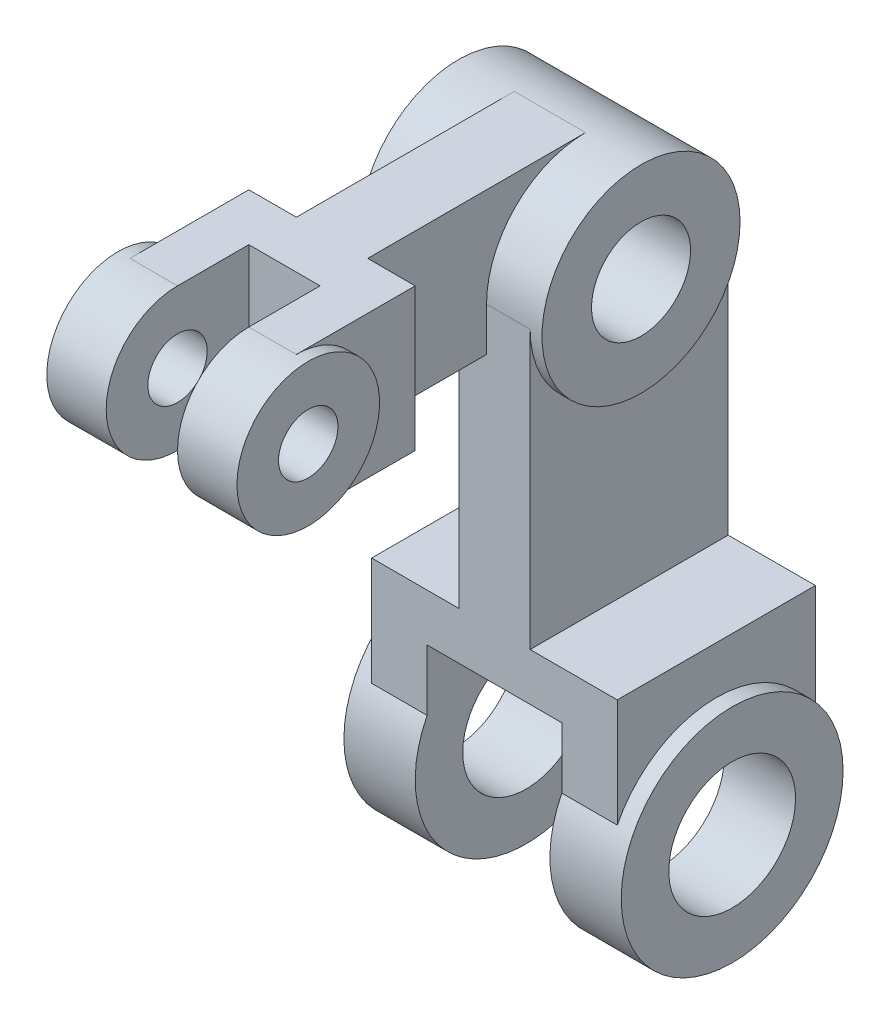
ISO-10303-21;
HEADER;
FILE_DESCRIPTION(('STEP AP214'),'2;1');
FILE_NAME('part.step','',(''),(''),'','','');
FILE_SCHEMA(('AUTOMOTIVE_DESIGN { 1 0 10303 214 1 1 1 1 }'));
ENDSEC;
DATA;
#1=APPLICATION_CONTEXT('core data for automotive mechanical design processes');
#2=APPLICATION_PROTOCOL_DEFINITION('international standard','automotive_design',2000,#1);
#3=PRODUCT_CONTEXT('',#1,'mechanical');
#4=PRODUCT('Part','Part','',(#3));
#5=PRODUCT_RELATED_PRODUCT_CATEGORY('part','',(#4));
#6=PRODUCT_DEFINITION_FORMATION('','',#4);
#7=PRODUCT_DEFINITION_CONTEXT('part definition',#1,'design');
#8=PRODUCT_DEFINITION('design','',#6,#7);
#9=PRODUCT_DEFINITION_SHAPE('','',#8);
#10=(LENGTH_UNIT() NAMED_UNIT(*) SI_UNIT(.MILLI.,.METRE.));
#11=(NAMED_UNIT(*) PLANE_ANGLE_UNIT() SI_UNIT($,.RADIAN.));
#12=(NAMED_UNIT(*) SI_UNIT($,.STERADIAN.) SOLID_ANGLE_UNIT());
#13=UNCERTAINTY_MEASURE_WITH_UNIT(LENGTH_MEASURE(1.E-05),#10,'distance_accuracy_value','');
#14=(GEOMETRIC_REPRESENTATION_CONTEXT(3) GLOBAL_UNCERTAINTY_ASSIGNED_CONTEXT((#13)) GLOBAL_UNIT_ASSIGNED_CONTEXT((#10,
#11,#12)) REPRESENTATION_CONTEXT('',''));
#15=CARTESIAN_POINT('',(0.,0.,0.));
#16=DIRECTION('',(0.,0.,1.));
#17=DIRECTION('',(1.,0.,0.));
#18=AXIS2_PLACEMENT_3D('',#15,#16,#17);
#19=CARTESIAN_POINT('',(-4.,40.,0.));
#20=DIRECTION('',(0.,1.,0.));
#21=DIRECTION('',(0.,0.,1.));
#22=AXIS2_PLACEMENT_3D('',#19,#20,#21);
#23=PLANE('',#22);
#24=DIRECTION('',(-1.,0.,0.));
#25=VECTOR('',#24,1.);
#26=CARTESIAN_POINT('',(-4.,40.,-25.));
#27=LINE('',#26,#25);
#28=CARTESIAN_POINT('',(-4.,40.,-25.));
#29=VERTEX_POINT('',#28);
#30=CARTESIAN_POINT('',(-26.,40.,-25.));
#31=VERTEX_POINT('',#30);
#32=EDGE_CURVE('E366',#29,#31,#27,.T.);
#33=ORIENTED_EDGE('',*,*,#32,.T.);
#34=DIRECTION('',(0.,0.,1.));
#35=VECTOR('',#34,1.);
#36=CARTESIAN_POINT('',(-26.,40.,-25.));
#37=LINE('',#36,#35);
#38=CARTESIAN_POINT('',(-26.,40.,25.));
#39=VERTEX_POINT('',#38);
#40=EDGE_CURVE('E286',#31,#39,#37,.T.);
#41=ORIENTED_EDGE('',*,*,#40,.T.);
#42=DIRECTION('',(-1.,0.,0.));
#43=VECTOR('',#42,1.);
#44=CARTESIAN_POINT('',(-4.,40.,25.));
#45=LINE('',#44,#43);
#46=CARTESIAN_POINT('',(-4.,40.,25.));
#47=VERTEX_POINT('',#46);
#48=EDGE_CURVE('E351',#47,#39,#45,.T.);
#49=ORIENTED_EDGE('',*,*,#48,.F.);
#50=DIRECTION('',(0.,0.,-1.));
#51=VECTOR('',#50,1.);
#52=CARTESIAN_POINT('',(-4.,40.,0.));
#53=LINE('',#52,#51);
#54=EDGE_CURVE('E344',#47,#29,#53,.T.);
#55=ORIENTED_EDGE('',*,*,#54,.T.);
#56=EDGE_LOOP('',(#33,#41,#49,#55));
#57=FACE_BOUND('',#56,.T.);
#58=ADVANCED_FACE('F44',(#57),#23,.T.);
#59=CARTESIAN_POINT('',(-18.,0.,0.));
#60=DIRECTION('',(1.,0.,0.));
#61=DIRECTION('',(0.,0.,-1.));
#62=AXIS2_PLACEMENT_3D('',#59,#60,#61);
#63=CYLINDRICAL_SURFACE('',#62,28.);
#64=DIRECTION('',(-1.,0.,0.));
#65=VECTOR('',#64,1.);
#66=CARTESIAN_POINT('',(-4.,12.6095202129185,25.));
#67=LINE('',#66,#65);
#68=CARTESIAN_POINT('',(-4.,12.6095202129185,25.));
#69=VERTEX_POINT('',#68);
#70=CARTESIAN_POINT('',(-18.,12.6095202129185,25.));
#71=VERTEX_POINT('',#70);
#72=EDGE_CURVE('E359',#69,#71,#67,.T.);
#73=ORIENTED_EDGE('',*,*,#72,.T.);
#74=CARTESIAN_POINT('',(-18.,0.,0.));
#75=DIRECTION('',(1.,0.,0.));
#76=DIRECTION('',(0.,0.,-1.));
#77=AXIS2_PLACEMENT_3D('',#74,#75,#76);
#78=CIRCLE('',#77,28.);
#79=CARTESIAN_POINT('',(-18.,12.6095202129185,-25.));
#80=VERTEX_POINT('',#79);
#81=EDGE_CURVE('E367',#71,#80,#78,.T.);
#82=ORIENTED_EDGE('',*,*,#81,.T.);
#83=DIRECTION('',(-1.,0.,0.));
#84=VECTOR('',#83,1.);
#85=CARTESIAN_POINT('',(-4.,12.6095202129185,-25.));
#86=LINE('',#85,#84);
#87=CARTESIAN_POINT('',(-4.,12.6095202129185,-25.));
#88=VERTEX_POINT('',#87);
#89=EDGE_CURVE('E361',#88,#80,#86,.T.);
#90=ORIENTED_EDGE('',*,*,#89,.F.);
#91=CARTESIAN_POINT('',(-4.,0.,0.));
#92=DIRECTION('',(1.,0.,0.));
#93=DIRECTION('',(0.,0.,1.));
#94=AXIS2_PLACEMENT_3D('',#91,#92,#93);
#95=CIRCLE('',#94,28.);
#96=EDGE_CURVE('E346',#88,#69,#95,.T.);
#97=ORIENTED_EDGE('',*,*,#96,.T.);
#98=EDGE_LOOP('',(#73,#82,#90,#97));
#99=FACE_BOUND('',#98,.T.);
#100=CARTESIAN_POINT('',(0.,0.,0.));
#101=DIRECTION('',(1.,0.,0.));
#102=DIRECTION('',(0.,0.,-1.));
#103=AXIS2_PLACEMENT_3D('',#100,#101,#102);
#104=CIRCLE('',#103,28.);
#105=CARTESIAN_POINT('',(0.,0.,-28.));
#106=VERTEX_POINT('',#105);
#107=EDGE_CURVE('E356',#106,#106,#104,.T.);
#108=ORIENTED_EDGE('',*,*,#107,.F.);
#109=EDGE_LOOP('',(#108));
#110=FACE_BOUND('',#109,.T.);
#111=ADVANCED_FACE('F50',(#99,#110),#63,.T.);
#112=CARTESIAN_POINT('',(-18.,0.,0.));
#113=DIRECTION('',(1.,0.,0.));
#114=DIRECTION('',(0.,0.,-1.));
#115=AXIS2_PLACEMENT_3D('',#112,#113,#114);
#116=PLANE('',#115);
#117=CARTESIAN_POINT('',(-18.,0.,0.));
#118=DIRECTION('',(1.,0.,0.));
#119=DIRECTION('',(0.,0.,-1.));
#120=AXIS2_PLACEMENT_3D('',#117,#118,#119);
#121=CIRCLE('',#120,16.);
#122=CARTESIAN_POINT('',(-18.,0.,-16.));
#123=VERTEX_POINT('',#122);
#124=EDGE_CURVE('E234',#123,#123,#121,.T.);
#125=ORIENTED_EDGE('',*,*,#124,.T.);
#126=EDGE_LOOP('',(#125));
#127=FACE_BOUND('',#126,.T.);
#128=ORIENTED_EDGE('',*,*,#81,.F.);
#129=DIRECTION('',(0.,1.,0.));
#130=VECTOR('',#129,1.);
#131=CARTESIAN_POINT('',(-18.,28.,25.));
#132=LINE('',#131,#130);
#133=CARTESIAN_POINT('',(-18.,28.,25.));
#134=VERTEX_POINT('',#133);
#135=EDGE_CURVE('E303',#71,#134,#132,.T.);
#136=ORIENTED_EDGE('',*,*,#135,.T.);
#137=DIRECTION('',(0.,0.,1.));
#138=VECTOR('',#137,1.);
#139=CARTESIAN_POINT('',(-18.,28.,-40.));
#140=LINE('',#139,#138);
#141=CARTESIAN_POINT('',(-18.,28.,-25.));
#142=VERTEX_POINT('',#141);
#143=EDGE_CURVE('E307',#142,#134,#140,.T.);
#144=ORIENTED_EDGE('',*,*,#143,.F.);
#145=DIRECTION('',(0.,-1.,0.));
#146=VECTOR('',#145,1.);
#147=CARTESIAN_POINT('',(-18.,40.,-25.));
#148=LINE('',#147,#146);
#149=EDGE_CURVE('E375',#142,#80,#148,.T.);
#150=ORIENTED_EDGE('',*,*,#149,.T.);
#151=EDGE_LOOP('',(#128,#136,#144,#150));
#152=FACE_BOUND('',#151,.T.);
#153=ADVANCED_FACE('F505',(#127,#152),#116,.F.);
#154=CARTESIAN_POINT('',(0.,0.,0.));
#155=DIRECTION('',(1.,0.,0.));
#156=DIRECTION('',(0.,0.,-1.));
#157=AXIS2_PLACEMENT_3D('',#154,#155,#156);
#158=PLANE('',#157);
#159=CARTESIAN_POINT('',(0.,0.,0.));
#160=DIRECTION('',(1.,0.,0.));
#161=DIRECTION('',(0.,0.,-1.));
#162=AXIS2_PLACEMENT_3D('',#159,#160,#161);
#163=CIRCLE('',#162,16.);
#164=CARTESIAN_POINT('',(0.,0.,-16.));
#165=VERTEX_POINT('',#164);
#166=EDGE_CURVE('E390',#165,#165,#163,.T.);
#167=ORIENTED_EDGE('',*,*,#166,.F.);
#168=EDGE_LOOP('',(#167));
#169=FACE_BOUND('',#168,.T.);
#170=ORIENTED_EDGE('',*,*,#107,.T.);
#171=EDGE_LOOP('',(#170));
#172=FACE_BOUND('',#171,.T.);
#173=ADVANCED_FACE('F570',(#169,#172),#158,.T.);
#174=DIRECTION('',(0.,0.,1.));
#175=VECTOR('',#174,1.);
#176=CARTESIAN_POINT('',(-44.,40.,-25.));
#177=LINE('',#176,#175);
#178=CARTESIAN_POINT('',(-44.,40.,-25.));
#179=VERTEX_POINT('',#178);
#180=CARTESIAN_POINT('',(-44.,40.,25.));
#181=VERTEX_POINT('',#180);
#182=EDGE_CURVE('E298',#179,#181,#177,.T.);
#183=ORIENTED_EDGE('',*,*,#182,.F.);
#184=CARTESIAN_POINT('',(-66.,40.,-25.));
#185=VERTEX_POINT('',#184);
#186=EDGE_CURVE('E355',#179,#185,#27,.T.);
#187=ORIENTED_EDGE('',*,*,#186,.T.);
#188=DIRECTION('',(0.,0.,-1.));
#189=VECTOR('',#188,1.);
#190=CARTESIAN_POINT('',(-66.,40.,0.));
#191=LINE('',#190,#189);
#192=CARTESIAN_POINT('',(-66.,40.,25.));
#193=VERTEX_POINT('',#192);
#194=EDGE_CURVE('E333',#193,#185,#191,.T.);
#195=ORIENTED_EDGE('',*,*,#194,.F.);
#196=EDGE_CURVE('E360',#181,#193,#45,.T.);
#197=ORIENTED_EDGE('',*,*,#196,.F.);
#198=EDGE_LOOP('',(#183,#187,#195,#197));
#199=FACE_BOUND('',#198,.T.);
#200=ADVANCED_FACE('F521',(#199),#23,.T.);
#201=CARTESIAN_POINT('',(-4.,40.,25.));
#202=DIRECTION('',(0.,0.,1.));
#203=DIRECTION('',(1.,0.,0.));
#204=AXIS2_PLACEMENT_3D('',#201,#202,#203);
#205=PLANE('',#204);
#206=DIRECTION('',(0.,1.,0.));
#207=VECTOR('',#206,1.);
#208=CARTESIAN_POINT('',(-37.,40.,25.));
#209=LINE('',#208,#207);
#210=CARTESIAN_POINT('',(-37.,99.,25.));
#211=VERTEX_POINT('',#210);
#212=CARTESIAN_POINT('',(-37.,110.,25.));
#213=VERTEX_POINT('',#212);
#214=EDGE_CURVE('E65',#211,#213,#209,.T.);
#215=ORIENTED_EDGE('',*,*,#214,.F.);
#216=DIRECTION('',(1.,0.,0.));
#217=VECTOR('',#216,1.);
#218=CARTESIAN_POINT('',(-4.,99.,25.));
#219=LINE('',#218,#217);
#220=CARTESIAN_POINT('',(-44.,99.,25.));
#221=VERTEX_POINT('',#220);
#222=EDGE_CURVE('E67',#221,#211,#219,.T.);
#223=ORIENTED_EDGE('',*,*,#222,.F.);
#224=DIRECTION('',(0.,-1.,0.));
#225=VECTOR('',#224,1.);
#226=CARTESIAN_POINT('',(-44.,110.,25.));
#227=LINE('',#226,#225);
#228=EDGE_CURVE('E283',#221,#181,#227,.T.);
#229=ORIENTED_EDGE('',*,*,#228,.T.);
#230=ORIENTED_EDGE('',*,*,#196,.T.);
#231=DIRECTION('',(0.,1.,0.));
#232=VECTOR('',#231,1.);
#233=CARTESIAN_POINT('',(-66.,40.,25.));
#234=LINE('',#233,#232);
#235=CARTESIAN_POINT('',(-66.,12.6095202129185,25.));
#236=VERTEX_POINT('',#235);
#237=EDGE_CURVE('E338',#236,#193,#234,.T.);
#238=ORIENTED_EDGE('',*,*,#237,.F.);
#239=DIRECTION('',(1.,0.,0.));
#240=VECTOR('',#239,1.);
#241=CARTESIAN_POINT('',(-70.,12.6095202129185,25.));
#242=LINE('',#241,#240);
#243=CARTESIAN_POINT('',(-52.,12.6095202129185,25.));
#244=VERTEX_POINT('',#243);
#245=EDGE_CURVE('E329',#236,#244,#242,.T.);
#246=ORIENTED_EDGE('',*,*,#245,.T.);
#247=DIRECTION('',(0.,-1.,0.));
#248=VECTOR('',#247,1.);
#249=CARTESIAN_POINT('',(-52.,12.6095202129185,25.));
#250=LINE('',#249,#248);
#251=CARTESIAN_POINT('',(-52.,28.,25.));
#252=VERTEX_POINT('',#251);
#253=EDGE_CURVE('E299',#252,#244,#250,.T.);
#254=ORIENTED_EDGE('',*,*,#253,.F.);
#255=DIRECTION('',(-1.,0.,0.));
#256=VECTOR('',#255,1.);
#257=CARTESIAN_POINT('',(-52.,28.,25.));
#258=LINE('',#257,#256);
#259=EDGE_CURVE('E306',#134,#252,#258,.T.);
#260=ORIENTED_EDGE('',*,*,#259,.F.);
#261=ORIENTED_EDGE('',*,*,#135,.F.);
#262=ORIENTED_EDGE('',*,*,#72,.F.);
#263=DIRECTION('',(0.,1.,0.));
#264=VECTOR('',#263,1.);
#265=CARTESIAN_POINT('',(-4.,40.,25.));
#266=LINE('',#265,#264);
#267=EDGE_CURVE('E353',#69,#47,#266,.T.);
#268=ORIENTED_EDGE('',*,*,#267,.T.);
#269=ORIENTED_EDGE('',*,*,#48,.T.);
#270=DIRECTION('',(0.,1.,0.));
#271=VECTOR('',#270,1.);
#272=CARTESIAN_POINT('',(-26.,40.,25.));
#273=LINE('',#272,#271);
#274=CARTESIAN_POINT('',(-26.,110.,25.));
#275=VERTEX_POINT('',#274);
#276=EDGE_CURVE('E282',#39,#275,#273,.T.);
#277=ORIENTED_EDGE('',*,*,#276,.T.);
#278=DIRECTION('',(-1.,0.,0.));
#279=VECTOR('',#278,1.);
#280=CARTESIAN_POINT('',(-26.,110.,25.));
#281=LINE('',#280,#279);
#282=EDGE_CURVE('E291',#275,#213,#281,.T.);
#283=ORIENTED_EDGE('',*,*,#282,.T.);
#284=EDGE_LOOP('',(#215,#223,#229,#230,#238,#246,#254,#260,#261,#262,#268,#269,#277,#283));
#285=FACE_BOUND('',#284,.T.);
#286=ADVANCED_FACE('F483',(#285),#205,.T.);
#287=CARTESIAN_POINT('',(-4.,40.,-25.));
#288=DIRECTION('',(0.,0.,-1.));
#289=DIRECTION('',(-1.,0.,0.));
#290=AXIS2_PLACEMENT_3D('',#287,#288,#289);
#291=PLANE('',#290);
#292=DIRECTION('',(0.,1.,0.));
#293=VECTOR('',#292,1.);
#294=CARTESIAN_POINT('',(-52.,40.,-25.));
#295=LINE('',#294,#293);
#296=CARTESIAN_POINT('',(-52.,12.6095202129185,-25.));
#297=VERTEX_POINT('',#296);
#298=CARTESIAN_POINT('',(-52.,28.,-25.));
#299=VERTEX_POINT('',#298);
#300=EDGE_CURVE('E317',#297,#299,#295,.T.);
#301=ORIENTED_EDGE('',*,*,#300,.F.);
#302=DIRECTION('',(1.,0.,0.));
#303=VECTOR('',#302,1.);
#304=CARTESIAN_POINT('',(-70.,12.6095202129185,-25.));
#305=LINE('',#304,#303);
#306=CARTESIAN_POINT('',(-66.,12.6095202129185,-25.));
#307=VERTEX_POINT('',#306);
#308=EDGE_CURVE('E324',#297,#307,#305,.F.);
#309=ORIENTED_EDGE('',*,*,#308,.T.);
#310=DIRECTION('',(0.,-1.,0.));
#311=VECTOR('',#310,1.);
#312=CARTESIAN_POINT('',(-66.,40.,-25.));
#313=LINE('',#312,#311);
#314=EDGE_CURVE('E335',#185,#307,#313,.T.);
#315=ORIENTED_EDGE('',*,*,#314,.F.);
#316=ORIENTED_EDGE('',*,*,#186,.F.);
#317=DIRECTION('',(0.,-1.,0.));
#318=VECTOR('',#317,1.);
#319=CARTESIAN_POINT('',(-44.,110.,-25.));
#320=LINE('',#319,#318);
#321=CARTESIAN_POINT('',(-44.,110.,-25.));
#322=VERTEX_POINT('',#321);
#323=EDGE_CURVE('E287',#322,#179,#320,.T.);
#324=ORIENTED_EDGE('',*,*,#323,.F.);
#325=DIRECTION('',(-1.,0.,0.));
#326=VECTOR('',#325,1.);
#327=CARTESIAN_POINT('',(-26.,110.,-25.));
#328=LINE('',#327,#326);
#329=CARTESIAN_POINT('',(-26.,110.,-25.));
#330=VERTEX_POINT('',#329);
#331=EDGE_CURVE('E281',#330,#322,#328,.T.);
#332=ORIENTED_EDGE('',*,*,#331,.F.);
#333=DIRECTION('',(0.,1.,0.));
#334=VECTOR('',#333,1.);
#335=CARTESIAN_POINT('',(-26.,40.,-25.));
#336=LINE('',#335,#334);
#337=EDGE_CURVE('E285',#31,#330,#336,.T.);
#338=ORIENTED_EDGE('',*,*,#337,.F.);
#339=ORIENTED_EDGE('',*,*,#32,.F.);
#340=DIRECTION('',(0.,-1.,0.));
#341=VECTOR('',#340,1.);
#342=CARTESIAN_POINT('',(-4.,40.,-25.));
#343=LINE('',#342,#341);
#344=EDGE_CURVE('E347',#29,#88,#343,.T.);
#345=ORIENTED_EDGE('',*,*,#344,.T.);
#346=ORIENTED_EDGE('',*,*,#89,.T.);
#347=ORIENTED_EDGE('',*,*,#149,.F.);
#348=DIRECTION('',(1.,0.,0.));
#349=VECTOR('',#348,1.);
#350=CARTESIAN_POINT('',(-4.,28.,-25.));
#351=LINE('',#350,#349);
#352=EDGE_CURVE('E315',#299,#142,#351,.T.);
#353=ORIENTED_EDGE('',*,*,#352,.F.);
#354=EDGE_LOOP('',(#301,#309,#315,#316,#324,#332,#338,#339,#345,#346,#347,#353));
#355=FACE_BOUND('',#354,.T.);
#356=ADVANCED_FACE('F490',(#355),#291,.T.);
#357=CARTESIAN_POINT('',(-4.,0.,0.));
#358=DIRECTION('',(-1.,0.,0.));
#359=DIRECTION('',(0.,0.,1.));
#360=AXIS2_PLACEMENT_3D('',#357,#358,#359);
#361=PLANE('',#360);
#362=ORIENTED_EDGE('',*,*,#54,.F.);
#363=ORIENTED_EDGE('',*,*,#267,.F.);
#364=ORIENTED_EDGE('',*,*,#96,.F.);
#365=ORIENTED_EDGE('',*,*,#344,.F.);
#366=EDGE_LOOP('',(#362,#363,#364,#365));
#367=FACE_BOUND('',#366,.T.);
#368=ADVANCED_FACE('F491',(#367),#361,.F.);
#369=CARTESIAN_POINT('',(-66.,0.,0.));
#370=DIRECTION('',(-1.,0.,0.));
#371=DIRECTION('',(0.,0.,1.));
#372=AXIS2_PLACEMENT_3D('',#369,#370,#371);
#373=PLANE('',#372);
#374=ORIENTED_EDGE('',*,*,#194,.T.);
#375=ORIENTED_EDGE('',*,*,#314,.T.);
#376=CARTESIAN_POINT('',(-66.,0.,0.));
#377=DIRECTION('',(1.,0.,0.));
#378=DIRECTION('',(0.,0.,1.));
#379=AXIS2_PLACEMENT_3D('',#376,#377,#378);
#380=CIRCLE('',#379,28.);
#381=EDGE_CURVE('E340',#307,#236,#380,.T.);
#382=ORIENTED_EDGE('',*,*,#381,.T.);
#383=ORIENTED_EDGE('',*,*,#237,.T.);
#384=EDGE_LOOP('',(#374,#375,#382,#383));
#385=FACE_BOUND('',#384,.T.);
#386=ADVANCED_FACE('F519',(#385),#373,.T.);
#387=CARTESIAN_POINT('',(-70.,0.,0.));
#388=DIRECTION('',(1.,0.,0.));
#389=DIRECTION('',(0.,0.,-1.));
#390=AXIS2_PLACEMENT_3D('',#387,#388,#389);
#391=CYLINDRICAL_SURFACE('',#390,28.);
#392=ORIENTED_EDGE('',*,*,#245,.F.);
#393=ORIENTED_EDGE('',*,*,#381,.F.);
#394=ORIENTED_EDGE('',*,*,#308,.F.);
#395=CARTESIAN_POINT('',(-52.,0.,0.));
#396=DIRECTION('',(-1.,0.,0.));
#397=DIRECTION('',(0.,0.,1.));
#398=AXIS2_PLACEMENT_3D('',#395,#396,#397);
#399=CIRCLE('',#398,28.);
#400=EDGE_CURVE('E316',#297,#244,#399,.T.);
#401=ORIENTED_EDGE('',*,*,#400,.T.);
#402=EDGE_LOOP('',(#392,#393,#394,#401));
#403=FACE_BOUND('',#402,.T.);
#404=CARTESIAN_POINT('',(-70.,0.,0.));
#405=DIRECTION('',(-1.,0.,0.));
#406=DIRECTION('',(0.,0.,1.));
#407=AXIS2_PLACEMENT_3D('',#404,#405,#406);
#408=CIRCLE('',#407,28.);
#409=CARTESIAN_POINT('',(-70.,0.,28.));
#410=VERTEX_POINT('',#409);
#411=EDGE_CURVE('E318',#410,#410,#408,.T.);
#412=ORIENTED_EDGE('',*,*,#411,.F.);
#413=EDGE_LOOP('',(#412));
#414=FACE_BOUND('',#413,.T.);
#415=ADVANCED_FACE('F515',(#403,#414),#391,.T.);
#416=CARTESIAN_POINT('',(-70.,0.,0.));
#417=DIRECTION('',(-1.,0.,0.));
#418=DIRECTION('',(0.,0.,1.));
#419=AXIS2_PLACEMENT_3D('',#416,#417,#418);
#420=PLANE('',#419);
#421=CARTESIAN_POINT('',(-70.,0.,0.));
#422=DIRECTION('',(-1.,0.,0.));
#423=DIRECTION('',(0.,0.,1.));
#424=AXIS2_PLACEMENT_3D('',#421,#422,#423);
#425=CIRCLE('',#424,16.);
#426=CARTESIAN_POINT('',(-70.,0.,16.));
#427=VERTEX_POINT('',#426);
#428=EDGE_CURVE('E387',#427,#427,#425,.T.);
#429=ORIENTED_EDGE('',*,*,#428,.F.);
#430=EDGE_LOOP('',(#429));
#431=FACE_BOUND('',#430,.T.);
#432=ORIENTED_EDGE('',*,*,#411,.T.);
#433=EDGE_LOOP('',(#432));
#434=FACE_BOUND('',#433,.T.);
#435=ADVANCED_FACE('F595',(#431,#434),#420,.T.);
#436=CARTESIAN_POINT('',(-52.,0.,0.));
#437=DIRECTION('',(-1.,0.,0.));
#438=DIRECTION('',(0.,0.,1.));
#439=AXIS2_PLACEMENT_3D('',#436,#437,#438);
#440=PLANE('',#439);
#441=CARTESIAN_POINT('',(-52.,0.,0.));
#442=DIRECTION('',(-1.,0.,0.));
#443=DIRECTION('',(0.,0.,1.));
#444=AXIS2_PLACEMENT_3D('',#441,#442,#443);
#445=CIRCLE('',#444,16.);
#446=CARTESIAN_POINT('',(-52.,0.,16.));
#447=VERTEX_POINT('',#446);
#448=EDGE_CURVE('E381',#447,#447,#445,.T.);
#449=ORIENTED_EDGE('',*,*,#448,.T.);
#450=EDGE_LOOP('',(#449));
#451=FACE_BOUND('',#450,.T.);
#452=ORIENTED_EDGE('',*,*,#400,.F.);
#453=ORIENTED_EDGE('',*,*,#300,.T.);
#454=DIRECTION('',(0.,0.,1.));
#455=VECTOR('',#454,1.);
#456=CARTESIAN_POINT('',(-52.,28.,-40.));
#457=LINE('',#456,#455);
#458=EDGE_CURVE('E309',#299,#252,#457,.T.);
#459=ORIENTED_EDGE('',*,*,#458,.T.);
#460=ORIENTED_EDGE('',*,*,#253,.T.);
#461=EDGE_LOOP('',(#452,#453,#459,#460));
#462=FACE_BOUND('',#461,.T.);
#463=ADVANCED_FACE('F509',(#451,#462),#440,.F.);
#464=CARTESIAN_POINT('',(-52.,28.,-40.));
#465=DIRECTION('',(0.,1.,0.));
#466=DIRECTION('',(0.,0.,1.));
#467=AXIS2_PLACEMENT_3D('',#464,#465,#466);
#468=PLANE('',#467);
#469=ORIENTED_EDGE('',*,*,#143,.T.);
#470=ORIENTED_EDGE('',*,*,#259,.T.);
#471=ORIENTED_EDGE('',*,*,#458,.F.);
#472=ORIENTED_EDGE('',*,*,#352,.T.);
#473=EDGE_LOOP('',(#469,#470,#471,#472));
#474=FACE_BOUND('',#473,.T.);
#475=ADVANCED_FACE('F510',(#474),#468,.F.);
#476=CARTESIAN_POINT('',(-44.,110.,-25.));
#477=DIRECTION('',(-1.,0.,0.));
#478=DIRECTION('',(0.,-1.,0.));
#479=AXIS2_PLACEMENT_3D('',#476,#477,#478);
#480=PLANE('',#479);
#481=DIRECTION('',(0.,0.,1.));
#482=VECTOR('',#481,1.);
#483=CARTESIAN_POINT('',(-44.,99.,-25.));
#484=LINE('',#483,#482);
#485=CARTESIAN_POINT('',(-44.,99.,22.4499443206437));
#486=VERTEX_POINT('',#485);
#487=EDGE_CURVE('E257',#486,#221,#484,.T.);
#488=ORIENTED_EDGE('',*,*,#487,.F.);
#489=CARTESIAN_POINT('',(-44.,110.,0.));
#490=DIRECTION('',(-1.,0.,0.));
#491=DIRECTION('',(0.,-1.,0.));
#492=AXIS2_PLACEMENT_3D('',#489,#490,#491);
#493=CIRCLE('',#492,25.);
#494=EDGE_CURVE('E279',#322,#486,#493,.T.);
#495=ORIENTED_EDGE('',*,*,#494,.F.);
#496=ORIENTED_EDGE('',*,*,#323,.T.);
#497=ORIENTED_EDGE('',*,*,#182,.T.);
#498=ORIENTED_EDGE('',*,*,#228,.F.);
#499=EDGE_LOOP('',(#488,#495,#496,#497,#498));
#500=FACE_BOUND('',#499,.T.);
#501=ADVANCED_FACE('F528',(#500),#480,.T.);
#502=CARTESIAN_POINT('',(-26.,40.,-25.));
#503=DIRECTION('',(1.,0.,0.));
#504=DIRECTION('',(0.,0.,-1.));
#505=AXIS2_PLACEMENT_3D('',#502,#503,#504);
#506=PLANE('',#505);
#507=CARTESIAN_POINT('',(-26.,110.,0.));
#508=DIRECTION('',(1.,0.,0.));
#509=DIRECTION('',(0.,0.,-1.));
#510=AXIS2_PLACEMENT_3D('',#507,#508,#509);
#511=CIRCLE('',#510,25.);
#512=EDGE_CURVE('E376',#275,#330,#511,.T.);
#513=ORIENTED_EDGE('',*,*,#512,.F.);
#514=ORIENTED_EDGE('',*,*,#276,.F.);
#515=ORIENTED_EDGE('',*,*,#40,.F.);
#516=ORIENTED_EDGE('',*,*,#337,.T.);
#517=EDGE_LOOP('',(#513,#514,#515,#516));
#518=FACE_BOUND('',#517,.T.);
#519=ADVANCED_FACE('F485',(#518),#506,.T.);
#520=CARTESIAN_POINT('',(-69.,110.,0.));
#521=DIRECTION('',(1.,0.,0.));
#522=DIRECTION('',(0.,0.,-1.));
#523=AXIS2_PLACEMENT_3D('',#520,#521,#522);
#524=CYLINDRICAL_SURFACE('',#523,25.);
#525=DIRECTION('',(1.,0.,0.));
#526=VECTOR('',#525,1.);
#527=CARTESIAN_POINT('',(-69.,99.,22.4499443206437));
#528=LINE('',#527,#526);
#529=CARTESIAN_POINT('',(-55.,99.,22.4499443206437));
#530=VERTEX_POINT('',#529);
#531=EDGE_CURVE('E11',#530,#486,#528,.T.);
#532=ORIENTED_EDGE('',*,*,#531,.F.);
#533=CARTESIAN_POINT('',(-55.,110.,0.));
#534=DIRECTION('',(-1.,0.,0.));
#535=DIRECTION('',(0.,0.,1.));
#536=AXIS2_PLACEMENT_3D('',#533,#534,#535);
#537=CIRCLE('',#536,25.);
#538=CARTESIAN_POINT('',(-55.,135.,0.));
#539=VERTEX_POINT('',#538);
#540=EDGE_CURVE('E378',#539,#530,#537,.F.);
#541=ORIENTED_EDGE('',*,*,#540,.F.);
#542=DIRECTION('',(-1.,0.,0.));
#543=VECTOR('',#542,1.);
#544=CARTESIAN_POINT('',(-55.,135.,0.));
#545=LINE('',#544,#543);
#546=CARTESIAN_POINT('',(-37.,135.,0.));
#547=VERTEX_POINT('',#546);
#548=EDGE_CURVE('E416',#547,#539,#545,.T.);
#549=ORIENTED_EDGE('',*,*,#548,.F.);
#550=CARTESIAN_POINT('',(-37.,110.,0.));
#551=DIRECTION('',(1.,0.,0.));
#552=DIRECTION('',(0.,0.,-1.));
#553=AXIS2_PLACEMENT_3D('',#550,#551,#552);
#554=CIRCLE('',#553,25.);
#555=EDGE_CURVE('E53',#213,#547,#554,.F.);
#556=ORIENTED_EDGE('',*,*,#555,.F.);
#557=ORIENTED_EDGE('',*,*,#282,.F.);
#558=ORIENTED_EDGE('',*,*,#512,.T.);
#559=ORIENTED_EDGE('',*,*,#331,.T.);
#560=ORIENTED_EDGE('',*,*,#494,.T.);
#561=EDGE_LOOP('',(#532,#541,#549,#556,#557,#558,#559,#560));
#562=FACE_BOUND('',#561,.T.);
#563=CARTESIAN_POINT('',(-69.,110.,0.));
#564=DIRECTION('',(1.,0.,0.));
#565=DIRECTION('',(0.,0.,-1.));
#566=AXIS2_PLACEMENT_3D('',#563,#564,#565);
#567=CIRCLE('',#566,25.);
#568=CARTESIAN_POINT('',(-69.,110.,-25.));
#569=VERTEX_POINT('',#568);
#570=EDGE_CURVE('E273',#569,#569,#567,.T.);
#571=ORIENTED_EDGE('',*,*,#570,.T.);
#572=EDGE_LOOP('',(#571));
#573=FACE_BOUND('',#572,.T.);
#574=CARTESIAN_POINT('',(-23.,110.,0.));
#575=DIRECTION('',(1.,0.,0.));
#576=DIRECTION('',(0.,0.,-1.));
#577=AXIS2_PLACEMENT_3D('',#574,#575,#576);
#578=CIRCLE('',#577,25.);
#579=CARTESIAN_POINT('',(-23.,110.,-25.));
#580=VERTEX_POINT('',#579);
#581=EDGE_CURVE('E275',#580,#580,#578,.T.);
#582=ORIENTED_EDGE('',*,*,#581,.F.);
#583=EDGE_LOOP('',(#582));
#584=FACE_BOUND('',#583,.T.);
#585=ADVANCED_FACE('F476',(#562,#573,#584),#524,.T.);
#586=CARTESIAN_POINT('',(-69.,110.,0.));
#587=DIRECTION('',(1.,0.,0.));
#588=DIRECTION('',(0.,0.,-1.));
#589=AXIS2_PLACEMENT_3D('',#586,#587,#588);
#590=PLANE('',#589);
#591=CARTESIAN_POINT('',(-69.,110.,0.));
#592=DIRECTION('',(-1.,0.,0.));
#593=DIRECTION('',(0.,0.,1.));
#594=AXIS2_PLACEMENT_3D('',#591,#592,#593);
#595=CIRCLE('',#594,12.5);
#596=CARTESIAN_POINT('',(-69.,110.,12.5));
#597=VERTEX_POINT('',#596);
#598=EDGE_CURVE('E388',#597,#597,#595,.T.);
#599=ORIENTED_EDGE('',*,*,#598,.F.);
#600=EDGE_LOOP('',(#599));
#601=FACE_BOUND('',#600,.T.);
#602=ORIENTED_EDGE('',*,*,#570,.F.);
#603=EDGE_LOOP('',(#602));
#604=FACE_BOUND('',#603,.T.);
#605=ADVANCED_FACE('F607',(#601,#604),#590,.F.);
#606=CARTESIAN_POINT('',(-23.,110.,0.));
#607=DIRECTION('',(1.,0.,0.));
#608=DIRECTION('',(0.,0.,-1.));
#609=AXIS2_PLACEMENT_3D('',#606,#607,#608);
#610=PLANE('',#609);
#611=CARTESIAN_POINT('',(-23.,110.,0.));
#612=DIRECTION('',(1.,0.,0.));
#613=DIRECTION('',(0.,0.,-1.));
#614=AXIS2_PLACEMENT_3D('',#611,#612,#613);
#615=CIRCLE('',#614,12.5);
#616=CARTESIAN_POINT('',(-23.,110.,-12.5));
#617=VERTEX_POINT('',#616);
#618=EDGE_CURVE('E389',#617,#617,#615,.T.);
#619=ORIENTED_EDGE('',*,*,#618,.F.);
#620=EDGE_LOOP('',(#619));
#621=FACE_BOUND('',#620,.T.);
#622=ORIENTED_EDGE('',*,*,#581,.T.);
#623=EDGE_LOOP('',(#622));
#624=FACE_BOUND('',#623,.T.);
#625=ADVANCED_FACE('F606',(#621,#624),#610,.T.);
#626=CARTESIAN_POINT('',(-37.,99.,0.));
#627=DIRECTION('',(1.,0.,0.));
#628=DIRECTION('',(0.,0.,-1.));
#629=AXIS2_PLACEMENT_3D('',#626,#627,#628);
#630=PLANE('',#629);
#631=DIRECTION('',(0.,0.,-1.));
#632=VECTOR('',#631,1.);
#633=CARTESIAN_POINT('',(-37.,99.,0.));
#634=LINE('',#633,#632);
#635=CARTESIAN_POINT('',(-37.,99.,55.));
#636=VERTEX_POINT('',#635);
#637=EDGE_CURVE('E269',#636,#211,#634,.T.);
#638=ORIENTED_EDGE('',*,*,#637,.T.);
#639=ORIENTED_EDGE('',*,*,#214,.T.);
#640=ORIENTED_EDGE('',*,*,#555,.T.);
#641=DIRECTION('',(0.,0.,-1.));
#642=VECTOR('',#641,1.);
#643=CARTESIAN_POINT('',(-37.,135.,0.));
#644=LINE('',#643,#642);
#645=CARTESIAN_POINT('',(-37.,135.,55.));
#646=VERTEX_POINT('',#645);
#647=EDGE_CURVE('E249',#646,#547,#644,.T.);
#648=ORIENTED_EDGE('',*,*,#647,.F.);
#649=DIRECTION('',(0.,1.,0.));
#650=VECTOR('',#649,1.);
#651=CARTESIAN_POINT('',(-37.,99.,55.));
#652=LINE('',#651,#650);
#653=EDGE_CURVE('E251',#636,#646,#652,.T.);
#654=ORIENTED_EDGE('',*,*,#653,.F.);
#655=EDGE_LOOP('',(#638,#639,#640,#648,#654));
#656=FACE_BOUND('',#655,.T.);
#657=ADVANCED_FACE('F477',(#656),#630,.T.);
#658=CARTESIAN_POINT('',(-37.,99.,55.));
#659=DIRECTION('',(0.,0.,-1.));
#660=DIRECTION('',(-1.,0.,0.));
#661=AXIS2_PLACEMENT_3D('',#658,#659,#660);
#662=PLANE('',#661);
#663=DIRECTION('',(-1.,0.,0.));
#664=VECTOR('',#663,1.);
#665=CARTESIAN_POINT('',(-37.,135.,55.));
#666=LINE('',#665,#664);
#667=CARTESIAN_POINT('',(-25.,135.,55.));
#668=VERTEX_POINT('',#667);
#669=EDGE_CURVE('E250',#668,#646,#666,.T.);
#670=ORIENTED_EDGE('',*,*,#669,.F.);
#671=DIRECTION('',(0.,1.,0.));
#672=VECTOR('',#671,1.);
#673=CARTESIAN_POINT('',(-25.,99.,55.));
#674=LINE('',#673,#672);
#675=CARTESIAN_POINT('',(-25.,99.,55.));
#676=VERTEX_POINT('',#675);
#677=EDGE_CURVE('E260',#676,#668,#674,.T.);
#678=ORIENTED_EDGE('',*,*,#677,.F.);
#679=DIRECTION('',(-1.,0.,0.));
#680=VECTOR('',#679,1.);
#681=CARTESIAN_POINT('',(-37.,99.,55.));
#682=LINE('',#681,#680);
#683=EDGE_CURVE('E445',#676,#636,#682,.T.);
#684=ORIENTED_EDGE('',*,*,#683,.T.);
#685=ORIENTED_EDGE('',*,*,#653,.T.);
#686=EDGE_LOOP('',(#670,#678,#684,#685));
#687=FACE_BOUND('',#686,.T.);
#688=ADVANCED_FACE('F628',(#687),#662,.T.);
#689=CARTESIAN_POINT('',(-25.,99.,55.));
#690=DIRECTION('',(1.,0.,0.));
#691=DIRECTION('',(0.,0.,-1.));
#692=AXIS2_PLACEMENT_3D('',#689,#690,#691);
#693=PLANE('',#692);
#694=CARTESIAN_POINT('',(-25.,117.,85.));
#695=DIRECTION('',(1.,0.,0.));
#696=DIRECTION('',(0.,0.,-1.));
#697=AXIS2_PLACEMENT_3D('',#694,#695,#696);
#698=CIRCLE('',#697,18.);
#699=CARTESIAN_POINT('',(-25.,99.,85.));
#700=VERTEX_POINT('',#699);
#701=CARTESIAN_POINT('',(-25.,135.,85.));
#702=VERTEX_POINT('',#701);
#703=EDGE_CURVE('E219',#700,#702,#698,.T.);
#704=ORIENTED_EDGE('',*,*,#703,.F.);
#705=DIRECTION('',(0.,0.,-1.));
#706=VECTOR('',#705,1.);
#707=CARTESIAN_POINT('',(-25.,99.,55.));
#708=LINE('',#707,#706);
#709=EDGE_CURVE('E437',#700,#676,#708,.T.);
#710=ORIENTED_EDGE('',*,*,#709,.T.);
#711=ORIENTED_EDGE('',*,*,#677,.T.);
#712=DIRECTION('',(0.,0.,-1.));
#713=VECTOR('',#712,1.);
#714=CARTESIAN_POINT('',(-25.,135.,55.));
#715=LINE('',#714,#713);
#716=EDGE_CURVE('E222',#702,#668,#715,.T.);
#717=ORIENTED_EDGE('',*,*,#716,.F.);
#718=EDGE_LOOP('',(#704,#710,#711,#717));
#719=FACE_BOUND('',#718,.T.);
#720=ADVANCED_FACE('F472',(#719),#693,.T.);
#721=CARTESIAN_POINT('',(-37.,99.,85.));
#722=DIRECTION('',(-1.,0.,0.));
#723=DIRECTION('',(0.,0.,1.));
#724=AXIS2_PLACEMENT_3D('',#721,#722,#723);
#725=PLANE('',#724);
#726=CARTESIAN_POINT('',(-37.,117.,85.));
#727=DIRECTION('',(-1.,0.,0.));
#728=DIRECTION('',(0.,0.,1.));
#729=AXIS2_PLACEMENT_3D('',#726,#727,#728);
#730=CIRCLE('',#729,7.50000000000001);
#731=CARTESIAN_POINT('',(-37.,117.,92.5));
#732=VERTEX_POINT('',#731);
#733=EDGE_CURVE('E398',#732,#732,#730,.T.);
#734=ORIENTED_EDGE('',*,*,#733,.F.);
#735=EDGE_LOOP('',(#734));
#736=FACE_BOUND('',#735,.T.);
#737=DIRECTION('',(0.,0.,1.));
#738=VECTOR('',#737,1.);
#739=CARTESIAN_POINT('',(-37.,99.,85.));
#740=LINE('',#739,#738);
#741=CARTESIAN_POINT('',(-37.,99.,67.));
#742=VERTEX_POINT('',#741);
#743=CARTESIAN_POINT('',(-37.,99.,85.));
#744=VERTEX_POINT('',#743);
#745=EDGE_CURVE('E235',#742,#744,#740,.T.);
#746=ORIENTED_EDGE('',*,*,#745,.T.);
#747=CARTESIAN_POINT('',(-37.,117.,85.));
#748=DIRECTION('',(-1.,0.,0.));
#749=DIRECTION('',(0.,0.,1.));
#750=AXIS2_PLACEMENT_3D('',#747,#748,#749);
#751=CIRCLE('',#750,18.);
#752=CARTESIAN_POINT('',(-37.,135.,85.));
#753=VERTEX_POINT('',#752);
#754=EDGE_CURVE('E213',#744,#753,#751,.T.);
#755=ORIENTED_EDGE('',*,*,#754,.T.);
#756=DIRECTION('',(0.,0.,1.));
#757=VECTOR('',#756,1.);
#758=CARTESIAN_POINT('',(-37.,135.,85.));
#759=LINE('',#758,#757);
#760=CARTESIAN_POINT('',(-37.,135.,67.));
#761=VERTEX_POINT('',#760);
#762=EDGE_CURVE('E225',#761,#753,#759,.T.);
#763=ORIENTED_EDGE('',*,*,#762,.F.);
#764=DIRECTION('',(0.,1.,0.));
#765=VECTOR('',#764,1.);
#766=CARTESIAN_POINT('',(-37.,99.,67.));
#767=LINE('',#766,#765);
#768=EDGE_CURVE('E256',#742,#761,#767,.T.);
#769=ORIENTED_EDGE('',*,*,#768,.F.);
#770=EDGE_LOOP('',(#746,#755,#763,#769));
#771=FACE_BOUND('',#770,.T.);
#772=ADVANCED_FACE('F230',(#736,#771),#725,.T.);
#773=CARTESIAN_POINT('',(-37.,99.,67.));
#774=DIRECTION('',(0.,0.,1.));
#775=DIRECTION('',(1.,0.,0.));
#776=AXIS2_PLACEMENT_3D('',#773,#774,#775);
#777=PLANE('',#776);
#778=DIRECTION('',(1.,0.,0.));
#779=VECTOR('',#778,1.);
#780=CARTESIAN_POINT('',(-37.,135.,67.));
#781=LINE('',#780,#779);
#782=CARTESIAN_POINT('',(-55.,135.,67.));
#783=VERTEX_POINT('',#782);
#784=EDGE_CURVE('E239',#783,#761,#781,.T.);
#785=ORIENTED_EDGE('',*,*,#784,.F.);
#786=DIRECTION('',(0.,1.,0.));
#787=VECTOR('',#786,1.);
#788=CARTESIAN_POINT('',(-55.,99.,67.));
#789=LINE('',#788,#787);
#790=CARTESIAN_POINT('',(-55.,99.,67.));
#791=VERTEX_POINT('',#790);
#792=EDGE_CURVE('E262',#791,#783,#789,.T.);
#793=ORIENTED_EDGE('',*,*,#792,.F.);
#794=DIRECTION('',(1.,0.,0.));
#795=VECTOR('',#794,1.);
#796=CARTESIAN_POINT('',(-37.,99.,67.));
#797=LINE('',#796,#795);
#798=EDGE_CURVE('E433',#791,#742,#797,.T.);
#799=ORIENTED_EDGE('',*,*,#798,.T.);
#800=ORIENTED_EDGE('',*,*,#768,.T.);
#801=EDGE_LOOP('',(#785,#793,#799,#800));
#802=FACE_BOUND('',#801,.T.);
#803=ADVANCED_FACE('F461',(#802),#777,.T.);
#804=CARTESIAN_POINT('',(-55.,99.,67.));
#805=DIRECTION('',(1.,0.,0.));
#806=DIRECTION('',(0.,0.,-1.));
#807=AXIS2_PLACEMENT_3D('',#804,#805,#806);
#808=PLANE('',#807);
#809=CARTESIAN_POINT('',(-55.,117.,85.));
#810=DIRECTION('',(1.,0.,0.));
#811=DIRECTION('',(0.,0.,-1.));
#812=AXIS2_PLACEMENT_3D('',#809,#810,#811);
#813=CIRCLE('',#812,7.50000000000001);
#814=CARTESIAN_POINT('',(-55.,117.,77.5));
#815=VERTEX_POINT('',#814);
#816=EDGE_CURVE('E402',#815,#815,#813,.T.);
#817=ORIENTED_EDGE('',*,*,#816,.F.);
#818=EDGE_LOOP('',(#817));
#819=FACE_BOUND('',#818,.T.);
#820=ORIENTED_EDGE('',*,*,#792,.T.);
#821=DIRECTION('',(0.,0.,-1.));
#822=VECTOR('',#821,1.);
#823=CARTESIAN_POINT('',(-55.,135.,67.));
#824=LINE('',#823,#822);
#825=CARTESIAN_POINT('',(-55.,135.,85.));
#826=VERTEX_POINT('',#825);
#827=EDGE_CURVE('E245',#826,#783,#824,.T.);
#828=ORIENTED_EDGE('',*,*,#827,.F.);
#829=CARTESIAN_POINT('',(-55.,117.,85.));
#830=DIRECTION('',(1.,0.,0.));
#831=DIRECTION('',(0.,0.,-1.));
#832=AXIS2_PLACEMENT_3D('',#829,#830,#831);
#833=CIRCLE('',#832,18.);
#834=CARTESIAN_POINT('',(-55.,99.,85.));
#835=VERTEX_POINT('',#834);
#836=EDGE_CURVE('E415',#826,#835,#833,.T.);
#837=ORIENTED_EDGE('',*,*,#836,.T.);
#838=DIRECTION('',(0.,0.,-1.));
#839=VECTOR('',#838,1.);
#840=CARTESIAN_POINT('',(-55.,99.,67.));
#841=LINE('',#840,#839);
#842=EDGE_CURVE('E427',#835,#791,#841,.T.);
#843=ORIENTED_EDGE('',*,*,#842,.T.);
#844=EDGE_LOOP('',(#820,#828,#837,#843));
#845=FACE_BOUND('',#844,.T.);
#846=ADVANCED_FACE('F463',(#819,#845),#808,.T.);
#847=CARTESIAN_POINT('',(-67.,99.,85.));
#848=DIRECTION('',(-1.,0.,0.));
#849=DIRECTION('',(0.,0.,1.));
#850=AXIS2_PLACEMENT_3D('',#847,#848,#849);
#851=PLANE('',#850);
#852=CARTESIAN_POINT('',(-67.,117.,85.));
#853=DIRECTION('',(-1.,0.,0.));
#854=DIRECTION('',(0.,0.,1.));
#855=AXIS2_PLACEMENT_3D('',#852,#853,#854);
#856=CIRCLE('',#855,18.);
#857=CARTESIAN_POINT('',(-67.,135.,85.));
#858=VERTEX_POINT('',#857);
#859=CARTESIAN_POINT('',(-67.,99.,85.));
#860=VERTEX_POINT('',#859);
#861=EDGE_CURVE('E418',#858,#860,#856,.T.);
#862=ORIENTED_EDGE('',*,*,#861,.F.);
#863=DIRECTION('',(0.,0.,1.));
#864=VECTOR('',#863,1.);
#865=CARTESIAN_POINT('',(-67.,135.,85.));
#866=LINE('',#865,#864);
#867=CARTESIAN_POINT('',(-67.,135.,55.));
#868=VERTEX_POINT('',#867);
#869=EDGE_CURVE('E451',#868,#858,#866,.T.);
#870=ORIENTED_EDGE('',*,*,#869,.F.);
#871=DIRECTION('',(0.,1.,0.));
#872=VECTOR('',#871,1.);
#873=CARTESIAN_POINT('',(-67.,99.,55.));
#874=LINE('',#873,#872);
#875=CARTESIAN_POINT('',(-67.,99.,55.));
#876=VERTEX_POINT('',#875);
#877=EDGE_CURVE('E264',#876,#868,#874,.T.);
#878=ORIENTED_EDGE('',*,*,#877,.F.);
#879=DIRECTION('',(0.,0.,1.));
#880=VECTOR('',#879,1.);
#881=CARTESIAN_POINT('',(-67.,99.,85.));
#882=LINE('',#881,#880);
#883=EDGE_CURVE('E424',#876,#860,#882,.T.);
#884=ORIENTED_EDGE('',*,*,#883,.T.);
#885=EDGE_LOOP('',(#862,#870,#878,#884));
#886=FACE_BOUND('',#885,.T.);
#887=ADVANCED_FACE('F538',(#886),#851,.T.);
#888=CARTESIAN_POINT('',(-67.,99.,55.));
#889=DIRECTION('',(0.,0.,-1.));
#890=DIRECTION('',(-1.,0.,0.));
#891=AXIS2_PLACEMENT_3D('',#888,#889,#890);
#892=PLANE('',#891);
#893=DIRECTION('',(-1.,0.,0.));
#894=VECTOR('',#893,1.);
#895=CARTESIAN_POINT('',(-67.,135.,55.));
#896=LINE('',#895,#894);
#897=CARTESIAN_POINT('',(-55.,135.,55.));
#898=VERTEX_POINT('',#897);
#899=EDGE_CURVE('E452',#898,#868,#896,.T.);
#900=ORIENTED_EDGE('',*,*,#899,.F.);
#901=DIRECTION('',(0.,1.,0.));
#902=VECTOR('',#901,1.);
#903=CARTESIAN_POINT('',(-55.,99.,55.));
#904=LINE('',#903,#902);
#905=CARTESIAN_POINT('',(-55.,99.,55.));
#906=VERTEX_POINT('',#905);
#907=EDGE_CURVE('E263',#906,#898,#904,.T.);
#908=ORIENTED_EDGE('',*,*,#907,.F.);
#909=DIRECTION('',(-1.,0.,0.));
#910=VECTOR('',#909,1.);
#911=CARTESIAN_POINT('',(-67.,99.,55.));
#912=LINE('',#911,#910);
#913=EDGE_CURVE('E422',#906,#876,#912,.T.);
#914=ORIENTED_EDGE('',*,*,#913,.T.);
#915=ORIENTED_EDGE('',*,*,#877,.T.);
#916=EDGE_LOOP('',(#900,#908,#914,#915));
#917=FACE_BOUND('',#916,.T.);
#918=ADVANCED_FACE('F537',(#917),#892,.T.);
#919=CARTESIAN_POINT('',(-55.,99.,55.));
#920=DIRECTION('',(-1.,0.,0.));
#921=DIRECTION('',(0.,0.,1.));
#922=AXIS2_PLACEMENT_3D('',#919,#920,#921);
#923=PLANE('',#922);
#924=DIRECTION('',(0.,0.,1.));
#925=VECTOR('',#924,1.);
#926=CARTESIAN_POINT('',(-55.,135.,55.));
#927=LINE('',#926,#925);
#928=EDGE_CURVE('E449',#539,#898,#927,.T.);
#929=ORIENTED_EDGE('',*,*,#928,.F.);
#930=ORIENTED_EDGE('',*,*,#540,.T.);
#931=DIRECTION('',(0.,0.,1.));
#932=VECTOR('',#931,1.);
#933=CARTESIAN_POINT('',(-55.,99.,55.));
#934=LINE('',#933,#932);
#935=EDGE_CURVE('E254',#530,#906,#934,.T.);
#936=ORIENTED_EDGE('',*,*,#935,.T.);
#937=ORIENTED_EDGE('',*,*,#907,.T.);
#938=EDGE_LOOP('',(#929,#930,#936,#937));
#939=FACE_BOUND('',#938,.T.);
#940=ADVANCED_FACE('F531',(#939),#923,.T.);
#941=CARTESIAN_POINT('',(0.,99.,0.));
#942=DIRECTION('',(0.,-1.,0.));
#943=DIRECTION('',(0.,0.,-1.));
#944=AXIS2_PLACEMENT_3D('',#941,#942,#943);
#945=PLANE('',#944);
#946=ORIENTED_EDGE('',*,*,#487,.T.);
#947=ORIENTED_EDGE('',*,*,#222,.T.);
#948=ORIENTED_EDGE('',*,*,#637,.F.);
#949=ORIENTED_EDGE('',*,*,#683,.F.);
#950=ORIENTED_EDGE('',*,*,#709,.F.);
#951=DIRECTION('',(1.,0.,0.));
#952=VECTOR('',#951,1.);
#953=CARTESIAN_POINT('',(-25.,99.,85.));
#954=LINE('',#953,#952);
#955=EDGE_CURVE('E440',#744,#700,#954,.T.);
#956=ORIENTED_EDGE('',*,*,#955,.F.);
#957=ORIENTED_EDGE('',*,*,#745,.F.);
#958=ORIENTED_EDGE('',*,*,#798,.F.);
#959=ORIENTED_EDGE('',*,*,#842,.F.);
#960=DIRECTION('',(1.,0.,0.));
#961=VECTOR('',#960,1.);
#962=CARTESIAN_POINT('',(-55.,99.,85.));
#963=LINE('',#962,#961);
#964=EDGE_CURVE('E426',#860,#835,#963,.T.);
#965=ORIENTED_EDGE('',*,*,#964,.F.);
#966=ORIENTED_EDGE('',*,*,#883,.F.);
#967=ORIENTED_EDGE('',*,*,#913,.F.);
#968=ORIENTED_EDGE('',*,*,#935,.F.);
#969=ORIENTED_EDGE('',*,*,#531,.T.);
#970=EDGE_LOOP('',(#946,#947,#948,#949,#950,#956,#957,#958,#959,#965,#966,#967,#968,#969));
#971=FACE_BOUND('',#970,.T.);
#972=ADVANCED_FACE('F470',(#971),#945,.T.);
#973=CARTESIAN_POINT('',(0.,135.,0.));
#974=DIRECTION('',(0.,-1.,0.));
#975=DIRECTION('',(0.,0.,-1.));
#976=AXIS2_PLACEMENT_3D('',#973,#974,#975);
#977=PLANE('',#976);
#978=ORIENTED_EDGE('',*,*,#548,.T.);
#979=ORIENTED_EDGE('',*,*,#928,.T.);
#980=ORIENTED_EDGE('',*,*,#899,.T.);
#981=ORIENTED_EDGE('',*,*,#869,.T.);
#982=DIRECTION('',(1.,0.,0.));
#983=VECTOR('',#982,1.);
#984=CARTESIAN_POINT('',(-55.,135.,85.));
#985=LINE('',#984,#983);
#986=EDGE_CURVE('E460',#858,#826,#985,.T.);
#987=ORIENTED_EDGE('',*,*,#986,.T.);
#988=ORIENTED_EDGE('',*,*,#827,.T.);
#989=ORIENTED_EDGE('',*,*,#784,.T.);
#990=ORIENTED_EDGE('',*,*,#762,.T.);
#991=DIRECTION('',(1.,0.,0.));
#992=VECTOR('',#991,1.);
#993=CARTESIAN_POINT('',(-25.,135.,85.));
#994=LINE('',#993,#992);
#995=EDGE_CURVE('E215',#753,#702,#994,.T.);
#996=ORIENTED_EDGE('',*,*,#995,.T.);
#997=ORIENTED_EDGE('',*,*,#716,.T.);
#998=ORIENTED_EDGE('',*,*,#669,.T.);
#999=ORIENTED_EDGE('',*,*,#647,.T.);
#1000=EDGE_LOOP('',(#978,#979,#980,#981,#987,#988,#989,#990,#996,#997,#998,#999));
#1001=FACE_BOUND('',#1000,.T.);
#1002=ADVANCED_FACE('F240',(#1001),#977,.F.);
#1003=CARTESIAN_POINT('',(-70.,117.,85.));
#1004=DIRECTION('',(1.,0.,0.));
#1005=DIRECTION('',(0.,0.,-1.));
#1006=AXIS2_PLACEMENT_3D('',#1003,#1004,#1005);
#1007=CYLINDRICAL_SURFACE('',#1006,18.);
#1008=CARTESIAN_POINT('',(-70.,117.,85.));
#1009=DIRECTION('',(1.,0.,0.));
#1010=DIRECTION('',(0.,0.,-1.));
#1011=AXIS2_PLACEMENT_3D('',#1008,#1009,#1010);
#1012=CIRCLE('',#1011,18.);
#1013=CARTESIAN_POINT('',(-70.,117.,67.));
#1014=VERTEX_POINT('',#1013);
#1015=EDGE_CURVE('E414',#1014,#1014,#1012,.T.);
#1016=ORIENTED_EDGE('',*,*,#1015,.T.);
#1017=EDGE_LOOP('',(#1016));
#1018=FACE_BOUND('',#1017,.T.);
#1019=ORIENTED_EDGE('',*,*,#861,.T.);
#1020=ORIENTED_EDGE('',*,*,#964,.T.);
#1021=ORIENTED_EDGE('',*,*,#836,.F.);
#1022=ORIENTED_EDGE('',*,*,#986,.F.);
#1023=EDGE_LOOP('',(#1019,#1020,#1021,#1022));
#1024=FACE_BOUND('',#1023,.T.);
#1025=ADVANCED_FACE('F544',(#1018,#1024),#1007,.T.);
#1026=CARTESIAN_POINT('',(-70.,117.,85.));
#1027=DIRECTION('',(1.,0.,0.));
#1028=DIRECTION('',(0.,0.,-1.));
#1029=AXIS2_PLACEMENT_3D('',#1026,#1027,#1028);
#1030=PLANE('',#1029);
#1031=CARTESIAN_POINT('',(-70.,117.,85.));
#1032=DIRECTION('',(-1.,0.,0.));
#1033=DIRECTION('',(0.,0.,1.));
#1034=AXIS2_PLACEMENT_3D('',#1031,#1032,#1033);
#1035=CIRCLE('',#1034,7.50000000000001);
#1036=CARTESIAN_POINT('',(-70.,117.,92.5));
#1037=VERTEX_POINT('',#1036);
#1038=EDGE_CURVE('E994',#1037,#1037,#1035,.T.);
#1039=ORIENTED_EDGE('',*,*,#1038,.F.);
#1040=EDGE_LOOP('',(#1039));
#1041=FACE_BOUND('',#1040,.T.);
#1042=ORIENTED_EDGE('',*,*,#1015,.F.);
#1043=EDGE_LOOP('',(#1042));
#1044=FACE_BOUND('',#1043,.T.);
#1045=ADVANCED_FACE('F543',(#1041,#1044),#1030,.F.);
#1046=CARTESIAN_POINT('',(-22.,117.,85.));
#1047=DIRECTION('',(-1.,0.,0.));
#1048=DIRECTION('',(0.,0.,1.));
#1049=AXIS2_PLACEMENT_3D('',#1046,#1047,#1048);
#1050=CYLINDRICAL_SURFACE('',#1049,18.);
#1051=CARTESIAN_POINT('',(-22.,117.,85.));
#1052=DIRECTION('',(-1.,0.,0.));
#1053=DIRECTION('',(0.,0.,1.));
#1054=AXIS2_PLACEMENT_3D('',#1051,#1052,#1053);
#1055=CIRCLE('',#1054,18.);
#1056=CARTESIAN_POINT('',(-22.,117.,103.));
#1057=VERTEX_POINT('',#1056);
#1058=EDGE_CURVE('E231',#1057,#1057,#1055,.T.);
#1059=ORIENTED_EDGE('',*,*,#1058,.T.);
#1060=EDGE_LOOP('',(#1059));
#1061=FACE_BOUND('',#1060,.T.);
#1062=ORIENTED_EDGE('',*,*,#955,.T.);
#1063=ORIENTED_EDGE('',*,*,#703,.T.);
#1064=ORIENTED_EDGE('',*,*,#995,.F.);
#1065=ORIENTED_EDGE('',*,*,#754,.F.);
#1066=EDGE_LOOP('',(#1062,#1063,#1064,#1065));
#1067=FACE_BOUND('',#1066,.T.);
#1068=ADVANCED_FACE('F211',(#1061,#1067),#1050,.T.);
#1069=CARTESIAN_POINT('',(-22.,117.,85.));
#1070=DIRECTION('',(-1.,0.,0.));
#1071=DIRECTION('',(0.,0.,1.));
#1072=AXIS2_PLACEMENT_3D('',#1069,#1070,#1071);
#1073=PLANE('',#1072);
#1074=CARTESIAN_POINT('',(-22.,117.,85.));
#1075=DIRECTION('',(-1.,0.,0.));
#1076=DIRECTION('',(0.,0.,1.));
#1077=AXIS2_PLACEMENT_3D('',#1074,#1075,#1076);
#1078=CIRCLE('',#1077,7.50000000000001);
#1079=CARTESIAN_POINT('',(-22.,117.,92.5));
#1080=VERTEX_POINT('',#1079);
#1081=EDGE_CURVE('E47',#1080,#1080,#1078,.T.);
#1082=ORIENTED_EDGE('',*,*,#1081,.T.);
#1083=EDGE_LOOP('',(#1082));
#1084=FACE_BOUND('',#1083,.T.);
#1085=ORIENTED_EDGE('',*,*,#1058,.F.);
#1086=EDGE_LOOP('',(#1085));
#1087=FACE_BOUND('',#1086,.T.);
#1088=ADVANCED_FACE('F652',(#1084,#1087),#1073,.F.);
#1089=CARTESIAN_POINT('',(-132.,0.,0.));
#1090=DIRECTION('',(1.,0.,0.));
#1091=DIRECTION('',(0.,0.,-1.));
#1092=AXIS2_PLACEMENT_3D('',#1089,#1090,#1091);
#1093=CYLINDRICAL_SURFACE('',#1092,16.);
#1094=ORIENTED_EDGE('',*,*,#428,.T.);
#1095=EDGE_LOOP('',(#1094));
#1096=FACE_BOUND('',#1095,.T.);
#1097=ORIENTED_EDGE('',*,*,#448,.F.);
#1098=EDGE_LOOP('',(#1097));
#1099=FACE_BOUND('',#1098,.T.);
#1100=ADVANCED_FACE('F697',(#1096,#1099),#1093,.F.);
#1101=ORIENTED_EDGE('',*,*,#166,.T.);
#1102=EDGE_LOOP('',(#1101));
#1103=FACE_BOUND('',#1102,.T.);
#1104=ORIENTED_EDGE('',*,*,#124,.F.);
#1105=EDGE_LOOP('',(#1104));
#1106=FACE_BOUND('',#1105,.T.);
#1107=ADVANCED_FACE('F704',(#1103,#1106),#1093,.F.);
#1108=CARTESIAN_POINT('',(63.,110.,0.));
#1109=DIRECTION('',(-1.,0.,0.));
#1110=DIRECTION('',(0.,0.,1.));
#1111=AXIS2_PLACEMENT_3D('',#1108,#1109,#1110);
#1112=CYLINDRICAL_SURFACE('',#1111,12.5);
#1113=ORIENTED_EDGE('',*,*,#618,.T.);
#1114=EDGE_LOOP('',(#1113));
#1115=FACE_BOUND('',#1114,.T.);
#1116=ORIENTED_EDGE('',*,*,#598,.T.);
#1117=EDGE_LOOP('',(#1116));
#1118=FACE_BOUND('',#1117,.T.);
#1119=ADVANCED_FACE('F716',(#1115,#1118),#1112,.F.);
#1120=CARTESIAN_POINT('',(62.,117.,85.));
#1121=DIRECTION('',(-1.,0.,0.));
#1122=DIRECTION('',(0.,0.,1.));
#1123=AXIS2_PLACEMENT_3D('',#1120,#1121,#1122);
#1124=CYLINDRICAL_SURFACE('',#1123,7.50000000000001);
#1125=ORIENTED_EDGE('',*,*,#733,.T.);
#1126=EDGE_LOOP('',(#1125));
#1127=FACE_BOUND('',#1126,.T.);
#1128=ORIENTED_EDGE('',*,*,#1081,.F.);
#1129=EDGE_LOOP('',(#1128));
#1130=FACE_BOUND('',#1129,.T.);
#1131=ADVANCED_FACE('F749',(#1127,#1130),#1124,.F.);
#1132=ORIENTED_EDGE('',*,*,#816,.T.);
#1133=EDGE_LOOP('',(#1132));
#1134=FACE_BOUND('',#1133,.T.);
#1135=ORIENTED_EDGE('',*,*,#1038,.T.);
#1136=EDGE_LOOP('',(#1135));
#1137=FACE_BOUND('',#1136,.T.);
#1138=ADVANCED_FACE('F799',(#1134,#1137),#1124,.F.);
#1139=CLOSED_SHELL('',(#58,#111,#153,#173,#200,#286,#356,#368,#386,#415,#435,#463,#475,#501,
#519,#585,#605,#625,#657,#688,#720,#772,#803,#846,#887,#918,#940,#972,#1002,#1025,#1045,#1068,
#1088,#1100,#1107,#1119,#1131,#1138));
#1140=MANIFOLD_SOLID_BREP('B2',#1139);
#1141=ADVANCED_BREP_SHAPE_REPRESENTATION('',(#18,#1140),#14);
#1142=SHAPE_DEFINITION_REPRESENTATION(#9,#1141);
ENDSEC;
END-ISO-10303-21;
